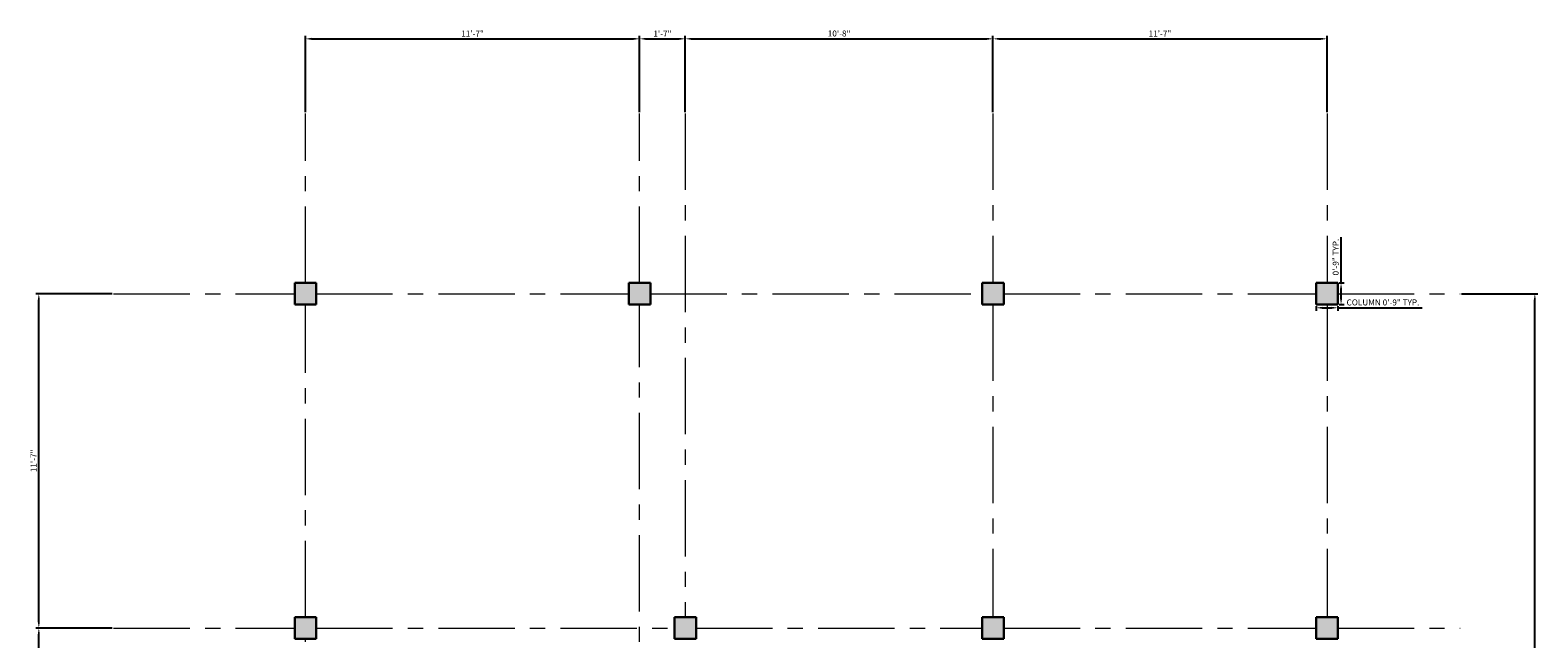
# Model space of a CAD drawing. Units: inches. Extents: x 4878 to 9282, y 5367 to 6617.
# Tile 14 of 14: x 8655 to 9282, y 6364 to 6617. Entities that reach past the tile are written whole.
import ezdxf

# ---------------------------------------------------------------- set-up
doc = ezdxf.new("R2010")
doc.units = ezdxf.units.IN
doc.linetypes.add('CENTER', pattern=[50.8, 31.75, -6.35, 6.35, -6.35])
for name, color, linetype, lineweight in [('A-ANNO-DIMS', 2, 'Continuous', 18), ('S-COLS', 1, 'Continuous', 30), ('S-COLS-PATT', 1, 'Continuous', 13), ('S-GRID', 4, 'CENTER', 13)]:
    doc.layers.add(name, color=color, linetype=linetype, lineweight=lineweight)
doc.styles.get("Standard").update_dxf_attribs({"font": 'arial.ttf'})
doc.dimstyles.new('ISO-25', dxfattribs={"dimtxt": 2.5, "dimasz": 2.5, "dimexe": 1.25, "dimexo": 0.625, "dimtad": 1, "dimdec": 0, "dimlunit": 3, "dimtxsty": 'Standard', "dimcen": 2.5, "dimadec": 0, "dimazin": 0, "dimtfac": 1, "dimtdec": 0, "dimtmove": 0, "dimatfit": 3, "dimfxl": 1, "dimarcsym": 0})

# ---------------------------------------------------------------- blocks, each defined once
blk = doc.blocks.new('COLUMN-9X9')
for p, q in [((0, 9), (9, 9)), ((0, 0), (0, 9)), ((9, 9), (9, 0)), ((0, 0), (9, 0))]:
    blk.add_line(p, q)
blk = doc.blocks.new('*D37')
at = {"layer": 'A-ANNO-DIMS', "color": 0, "lineweight": -2, "transparency": 16777216}
for p, q in [((9189.96, 6502.15), (9189.96, 6500.17)), ((9192.46, 6501.42), (9196.46, 6501.42)), ((9198.96, 6502.15), (9198.96, 6500.17)), ((9198.96, 6501.42), (9234.02, 6501.42))]:
    blk.add_line(p, q, dxfattribs=at)
at = {"layer": 'A-ANNO-DIMS', "color": 0, "transparency": 16777216}
for points in [[(9192.46, 6501.84), (9192.46, 6501), (9189.96, 6501.42)], [(9196.46, 6501.84), (9196.46, 6501), (9198.96, 6501.42)]]:
    blk.add_solid(points, dxfattribs=at)
at = {"layer": 'Defpoints', "color": 0, "transparency": 16777216}
for p in [(9189.96, 6502.77), (9198.96, 6502.77), (9198.96, 6501.42)]:
    blk.add_point(p, dxfattribs=at)
at = {"layer": 'A-ANNO-DIMS', "color": 0, "transparency": 16777216, "insert": (9217.74, 6503.34), "char_height": 2.5, "attachment_point": 5}
blk.add_mtext('COLUMN 0\'-9" TYP.', dxfattribs=at)
blk = doc.blocks.new('*D38')
at = {"layer": 'A-ANNO-DIMS', "color": 0, "lineweight": -2, "transparency": 16777216}
for p, q in [((9200.31, 6511.77), (9200.31, 6530.76)), ((9199.58, 6511.77), (9201.56, 6511.77)), ((9200.31, 6505.27), (9200.31, 6509.27)), ((9199.58, 6502.77), (9201.56, 6502.77))]:
    blk.add_line(p, q, dxfattribs=at)
at = {"layer": 'A-ANNO-DIMS', "color": 0, "transparency": 16777216}
for points in [[(9199.89, 6509.27), (9200.73, 6509.27), (9200.31, 6511.77)], [(9199.89, 6505.27), (9200.73, 6505.27), (9200.31, 6502.77)]]:
    blk.add_solid(points, dxfattribs=at)
at = {"layer": 'Defpoints', "color": 0, "transparency": 16777216}
for p in [(9198.96, 6511.77), (9200.31, 6511.77), (9198.96, 6502.77)]:
    blk.add_point(p, dxfattribs=at)
at = {"layer": 'A-ANNO-DIMS', "color": 0, "transparency": 16777216, "insert": (9198.41, 6522.52), "char_height": 2.5, "attachment_point": 5, "rotation": 90}
blk.add_mtext('0\'-9" TYP.', dxfattribs=at)
blk = doc.blocks.new('*D79')
at = {"layer": 'A-ANNO-DIMS', "color": 0, "lineweight": -2, "transparency": 16777216}
for p, q in [((8769.46, 6582.8), (8769.46, 6614.53)), ((8771.96, 6613.28), (8905.96, 6613.28)), ((8908.46, 6582.8), (8908.46, 6614.53))]:
    blk.add_line(p, q, dxfattribs=at)
at = {"layer": 'A-ANNO-DIMS', "color": 0, "transparency": 16777216}
for points in [[(8771.96, 6613.7), (8771.96, 6612.86), (8769.46, 6613.28)], [(8905.96, 6613.7), (8905.96, 6612.86), (8908.46, 6613.28)]]:
    blk.add_solid(points, dxfattribs=at)
at = {"layer": 'Defpoints', "color": 0, "transparency": 16777216}
for p in [(8908.46, 6613.28), (8769.46, 6582.18), (8908.46, 6582.18)]:
    blk.add_point(p, dxfattribs=at)
at = {"layer": 'A-ANNO-DIMS', "color": 0, "transparency": 16777216, "insert": (8838.96, 6615.16), "char_height": 2.5, "attachment_point": 5}
blk.add_mtext('11\'-7"', dxfattribs=at)
blk = doc.blocks.new('*D80')
at = {"layer": 'A-ANNO-DIMS', "color": 0, "lineweight": -2, "transparency": 16777216}
for p, q in [((8908.46, 6582.8), (8908.46, 6614.53)), ((8910.96, 6613.28), (8924.96, 6613.28)), ((8927.46, 6582.8), (8927.46, 6614.53))]:
    blk.add_line(p, q, dxfattribs=at)
at = {"layer": 'A-ANNO-DIMS', "color": 0, "transparency": 16777216}
for points in [[(8910.96, 6613.7), (8910.96, 6612.86), (8908.46, 6613.28)], [(8924.96, 6613.7), (8924.96, 6612.86), (8927.46, 6613.28)]]:
    blk.add_solid(points, dxfattribs=at)
at = {"layer": 'Defpoints', "color": 0, "transparency": 16777216}
for p in [(8927.46, 6613.28), (8908.46, 6582.18), (8927.46, 6582.18)]:
    blk.add_point(p, dxfattribs=at)
at = {"layer": 'A-ANNO-DIMS', "color": 0, "transparency": 16777216, "insert": (8917.96, 6615.16), "char_height": 2.5, "attachment_point": 5}
blk.add_mtext('1\'-7"', dxfattribs=at)
blk = doc.blocks.new('*D81')
at = {"layer": 'A-ANNO-DIMS', "color": 0, "lineweight": -2, "transparency": 16777216}
for p, q in [((8927.46, 6582.8), (8927.46, 6614.53)), ((8929.96, 6613.28), (9052.96, 6613.28)), ((9055.46, 6582.8), (9055.46, 6614.53))]:
    blk.add_line(p, q, dxfattribs=at)
at = {"layer": 'A-ANNO-DIMS', "color": 0, "transparency": 16777216}
for points in [[(8929.96, 6613.7), (8929.96, 6612.86), (8927.46, 6613.28)], [(9052.96, 6613.7), (9052.96, 6612.86), (9055.46, 6613.28)]]:
    blk.add_solid(points, dxfattribs=at)
at = {"layer": 'Defpoints', "color": 0, "transparency": 16777216}
for p in [(9055.46, 6613.28), (8927.46, 6582.18), (9055.46, 6582.18)]:
    blk.add_point(p, dxfattribs=at)
at = {"layer": 'A-ANNO-DIMS', "color": 0, "transparency": 16777216, "insert": (8991.46, 6615.18), "char_height": 2.5, "attachment_point": 5}
blk.add_mtext('10\'-8"', dxfattribs=at)
blk = doc.blocks.new('*D82')
at = {"layer": 'A-ANNO-DIMS', "color": 0, "lineweight": -2, "transparency": 16777216}
for p, q in [((9055.46, 6582.8), (9055.46, 6614.53)), ((9057.96, 6613.28), (9191.96, 6613.28)), ((9194.46, 6582.8), (9194.46, 6614.53))]:
    blk.add_line(p, q, dxfattribs=at)
at = {"layer": 'A-ANNO-DIMS', "color": 0, "transparency": 16777216}
for points in [[(9057.96, 6613.7), (9057.96, 6612.86), (9055.46, 6613.28)], [(9191.96, 6613.7), (9191.96, 6612.86), (9194.46, 6613.28)]]:
    blk.add_solid(points, dxfattribs=at)
at = {"layer": 'Defpoints', "color": 0, "transparency": 16777216}
for p in [(9194.46, 6613.28), (9055.46, 6582.18), (9194.46, 6582.18)]:
    blk.add_point(p, dxfattribs=at)
at = {"layer": 'A-ANNO-DIMS', "color": 0, "transparency": 16777216, "insert": (9124.96, 6615.16), "char_height": 2.5, "attachment_point": 5}
blk.add_mtext('11\'-7"', dxfattribs=at)
blk = doc.blocks.new('*D85')
at = {"layer": 'A-ANNO-DIMS', "color": 0, "lineweight": -2, "transparency": 16777216}
for p, q in [((8688.98, 6368.27), (8657.25, 6368.27)), ((8658.5, 6220.77), (8658.5, 6365.77)), ((8688.98, 6218.27), (8657.25, 6218.27))]:
    blk.add_line(p, q, dxfattribs=at)
at = {"layer": 'A-ANNO-DIMS', "color": 0, "transparency": 16777216}
for points in [[(8658.08, 6365.77), (8658.92, 6365.77), (8658.5, 6368.27)], [(8658.08, 6220.77), (8658.92, 6220.77), (8658.5, 6218.27)]]:
    blk.add_solid(points, dxfattribs=at)
at = {"layer": 'Defpoints', "color": 0, "transparency": 16777216}
for p in [(8658.5, 6368.27), (8689.6, 6368.27), (8689.6, 6218.27)]:
    blk.add_point(p, dxfattribs=at)
at = {"layer": 'A-ANNO-DIMS', "color": 0, "transparency": 16777216, "insert": (8656.6, 6293.27), "char_height": 2.5, "attachment_point": 5, "rotation": 90}
blk.add_mtext('12\'-6"', dxfattribs=at)
blk = doc.blocks.new('*D86')
at = {"layer": 'A-ANNO-DIMS', "color": 0, "lineweight": -2, "transparency": 16777216}
for p, q in [((8688.98, 6507.27), (8657.25, 6507.27)), ((8658.5, 6370.77), (8658.5, 6504.77)), ((8688.98, 6368.27), (8657.25, 6368.27))]:
    blk.add_line(p, q, dxfattribs=at)
at = {"layer": 'A-ANNO-DIMS', "color": 0, "transparency": 16777216}
for points in [[(8658.08, 6504.77), (8658.92, 6504.77), (8658.5, 6507.27)], [(8658.08, 6370.77), (8658.92, 6370.77), (8658.5, 6368.27)]]:
    blk.add_solid(points, dxfattribs=at)
at = {"layer": 'Defpoints', "color": 0, "transparency": 16777216}
for p in [(8658.5, 6507.27), (8689.6, 6507.27), (8689.6, 6368.27)]:
    blk.add_point(p, dxfattribs=at)
at = {"layer": 'A-ANNO-DIMS', "color": 0, "transparency": 16777216, "insert": (8656.62, 6437.77), "char_height": 2.5, "attachment_point": 5, "rotation": 90}
blk.add_mtext('11\'-7"', dxfattribs=at)
blk = doc.blocks.new('*D87')
at = {"layer": 'A-ANNO-DIMS', "color": 0, "lineweight": -2, "transparency": 16777216}
for p, q in [((9250.46, 6507.27), (9282.18, 6507.27)), ((9280.93, 6070.77), (9280.93, 6504.77)), ((9250.46, 6068.27), (9282.18, 6068.27))]:
    blk.add_line(p, q, dxfattribs=at)
at = {"layer": 'A-ANNO-DIMS', "color": 0, "transparency": 16777216}
for points in [[(9280.52, 6504.77), (9281.35, 6504.77), (9280.93, 6507.27)], [(9280.52, 6070.77), (9281.35, 6070.77), (9280.93, 6068.27)]]:
    blk.add_solid(points, dxfattribs=at)
at = {"layer": 'Defpoints', "color": 0, "transparency": 16777216}
for p in [(9249.83, 6507.27), (9280.93, 6507.27), (9249.83, 6068.27)]:
    blk.add_point(p, dxfattribs=at)
at = {"layer": 'A-ANNO-DIMS', "color": 0, "transparency": 16777216, "insert": (9279.03, 6287.77), "char_height": 2.5, "attachment_point": 5, "rotation": 90}
blk.add_mtext('36\'-7"', dxfattribs=at)

msp = doc.modelspace()

# ---------------------------------------------------------------- hatches: boundary and pattern name
at = {"layer": 'S-COLS-PATT'}
h = msp.add_hatch(color=256, dxfattribs=at)
h.dxf.hatch_style = 1
h.paths.add_polyline_path([(8931.96, 6072.77), (8922.96, 6072.77), (8922.96, 6063.77), (8931.96, 6063.77)])
h.paths.add_polyline_path([(9059.96, 6072.77), (9050.96, 6072.77), (9050.96, 6063.77), (9059.96, 6063.77)])
h.paths.add_polyline_path([(9198.96, 6072.77), (9189.96, 6072.77), (9189.96, 6063.77), (9198.96, 6063.77)])
h.paths.add_polyline_path([(9198.96, 6222.77), (9189.96, 6222.77), (9189.96, 6213.77), (9198.96, 6213.77)])
h.paths.add_polyline_path([(9059.96, 6222.77), (9050.96, 6222.77), (9050.96, 6213.77), (9059.96, 6213.77)])
h.paths.add_polyline_path([(8912.96, 6222.77), (8903.96, 6222.77), (8903.96, 6213.77), (8912.96, 6213.77)])
h.paths.add_polyline_path([(8773.96, 6222.77), (8764.96, 6222.77), (8764.96, 6213.77), (8773.96, 6213.77)])
h.paths.add_polyline_path([(8773.96, 6372.77), (8764.96, 6372.77), (8764.96, 6363.77), (8773.96, 6363.77)])
h.paths.add_polyline_path([(8931.96, 6372.77), (8922.96, 6372.77), (8922.96, 6363.77), (8931.96, 6363.77)])
h.paths.add_polyline_path([(9059.96, 6372.77), (9050.96, 6372.77), (9050.96, 6363.77), (9059.96, 6363.77)])
h.paths.add_polyline_path([(9198.96, 6372.77), (9189.96, 6372.77), (9189.96, 6363.77), (9198.96, 6363.77)])
h.paths.add_polyline_path([(9198.96, 6511.77), (9189.96, 6511.77), (9189.96, 6502.77), (9198.96, 6502.77)])
h.paths.add_polyline_path([(9059.96, 6511.77), (9050.96, 6511.77), (9050.96, 6502.77), (9059.96, 6502.77)])
h.paths.add_polyline_path([(8912.96, 6511.77), (8903.96, 6511.77), (8903.96, 6502.77), (8912.96, 6502.77)])
h.paths.add_polyline_path([(8773.96, 6511.77), (8764.96, 6511.77), (8764.96, 6502.77), (8773.96, 6502.77)])

# ---------------------------------------------------------------- linework, layer by layer
at = {"layer": 'S-COLS'}
for p, q in [((8773.96, 6372.77), (8773.96, 6363.77)), ((9050.96, 6372.77), (9059.96, 6372.77))]:
    msp.add_line(p, q, dxfattribs=at)
at = {"layer": 'S-GRID'}
for p, q in [((8769.46, 6511.77), (8769.46, 6582.18)), ((8908.46, 6511.77), (8908.46, 6582.18)), ((8927.46, 6582.18), (8927.46, 6372.77)), ((9055.46, 6582.18), (9055.46, 6511.77)), ((9194.46, 6582.18), (9194.46, 6511.77)), ((8689.6, 6507.27), (8764.96, 6507.27)), ((8773.96, 6507.27), (8903.96, 6507.27)), ((8912.96, 6507.27), (9050.96, 6507.27)), ((9059.96, 6507.27), (9189.96, 6507.27)), ((9198.96, 6507.27), (9249.83, 6507.27)), ((8769.46, 6372.77), (8769.46, 6502.77)), ((8908.46, 6222.77), (8908.46, 6502.77)), ((9055.46, 6502.77), (9055.46, 6372.77)), ((9194.46, 6502.77), (9194.46, 6372.77)), ((8689.6, 6368.27), (8764.96, 6368.27)), ((8773.96, 6368.27), (8922.96, 6368.27)), ((8931.96, 6368.27), (9050.96, 6368.27)), ((9059.96, 6368.27), (9189.96, 6368.27)), ((9198.96, 6368.27), (9249.83, 6368.27)), ((8769.46, 6222.77), (8769.46, 6363.77))]:
    msp.add_line(p, q, dxfattribs=at)

# ---------------------------------------------------------------- block references
at = {"layer": 'S-COLS'}
for p in [(8764.96, 6502.77), (8903.96, 6502.77), (9050.96, 6502.77), (9189.96, 6502.77), (8764.96, 6363.77), (8922.96, 6363.77), (9050.96, 6363.77), (9189.96, 6363.77)]:
    msp.add_blockref('COLUMN-9X9', p, dxfattribs=at)

# ---------------------------------------------------------------- dimensions: what is measured, and where the dimension line sits
at = {"layer": 'A-ANNO-DIMS'}
for base, p1, p2, picture, middle in [((8908.46, 6613.28), (8769.46, 6582.18), (8908.46, 6582.18), '*D79', (8838.96, 6615.16)), ((8927.46, 6613.28), (8908.46, 6582.18), (8927.46, 6582.18), '*D80', (8917.96, 6615.16)), ((9055.46, 6613.28), (8927.46, 6582.18), (9055.46, 6582.18), '*D81', (8991.46, 6615.18)), ((9194.46, 6613.28), (9055.46, 6582.18), (9194.46, 6582.18), '*D82', (9124.96, 6615.16))]:
    dim = msp.add_linear_dim(base=base, p1=p1, p2=p2, dimstyle='ISO-25', override={"dimdec": 1, "dimlfac": 1, "dimrnd": 0, "dimzin": 1, "dimdsep": 46, "dimlunit": 4, "dimfrac": 2}, dxfattribs=at)
    dim.commit()
    dim.dimension.update_dxf_attribs({"geometry": picture, "text_midpoint": middle})
dim = msp.add_linear_dim(base=(9200.31, 6511.77), p1=(9198.96, 6502.77), p2=(9198.96, 6511.77), angle=90, text='<> TYP.', dimstyle='ISO-25', override={"dimdec": 1, "dimlfac": 1, "dimrnd": 0, "dimzin": 1, "dimdsep": 46, "dimlunit": 4, "dimfrac": 2}, dxfattribs=at)
dim.commit()
dim.dimension.update_dxf_attribs({"geometry": '*D38', "text_midpoint": (9198.41, 6522.52)})
for base, p1, p2, picture, middle in [((8658.5, 6507.27), (8689.6, 6368.27), (8689.6, 6507.27), '*D86', (8656.62, 6437.77)), ((9280.93, 6507.27), (9249.83, 6068.27), (9249.83, 6507.27), '*D87', (9279.03, 6287.77)), ((8658.5, 6368.27), (8689.6, 6218.27), (8689.6, 6368.27), '*D85', (8656.6, 6293.27))]:
    dim = msp.add_linear_dim(base=base, p1=p1, p2=p2, angle=90, dimstyle='ISO-25', override={"dimdec": 1, "dimlfac": 1, "dimrnd": 0, "dimzin": 1, "dimdsep": 46, "dimlunit": 4, "dimfrac": 2}, dxfattribs=at)
    dim.commit()
    dim.dimension.update_dxf_attribs({"geometry": picture, "text_midpoint": middle})
dim = msp.add_linear_dim(base=(9198.96, 6501.42), p1=(9189.96, 6502.77), p2=(9198.96, 6502.77), text='COLUMN <> TYP.', dimstyle='ISO-25', override={"dimdec": 1, "dimlfac": 1, "dimrnd": 0, "dimzin": 1, "dimdsep": 46, "dimlunit": 4, "dimfrac": 2}, dxfattribs=at)
dim.commit()
dim.dimension.update_dxf_attribs({"geometry": '*D37', "text_midpoint": (9217.74, 6503.34)})

doc.saveas('drawing.dxf')
